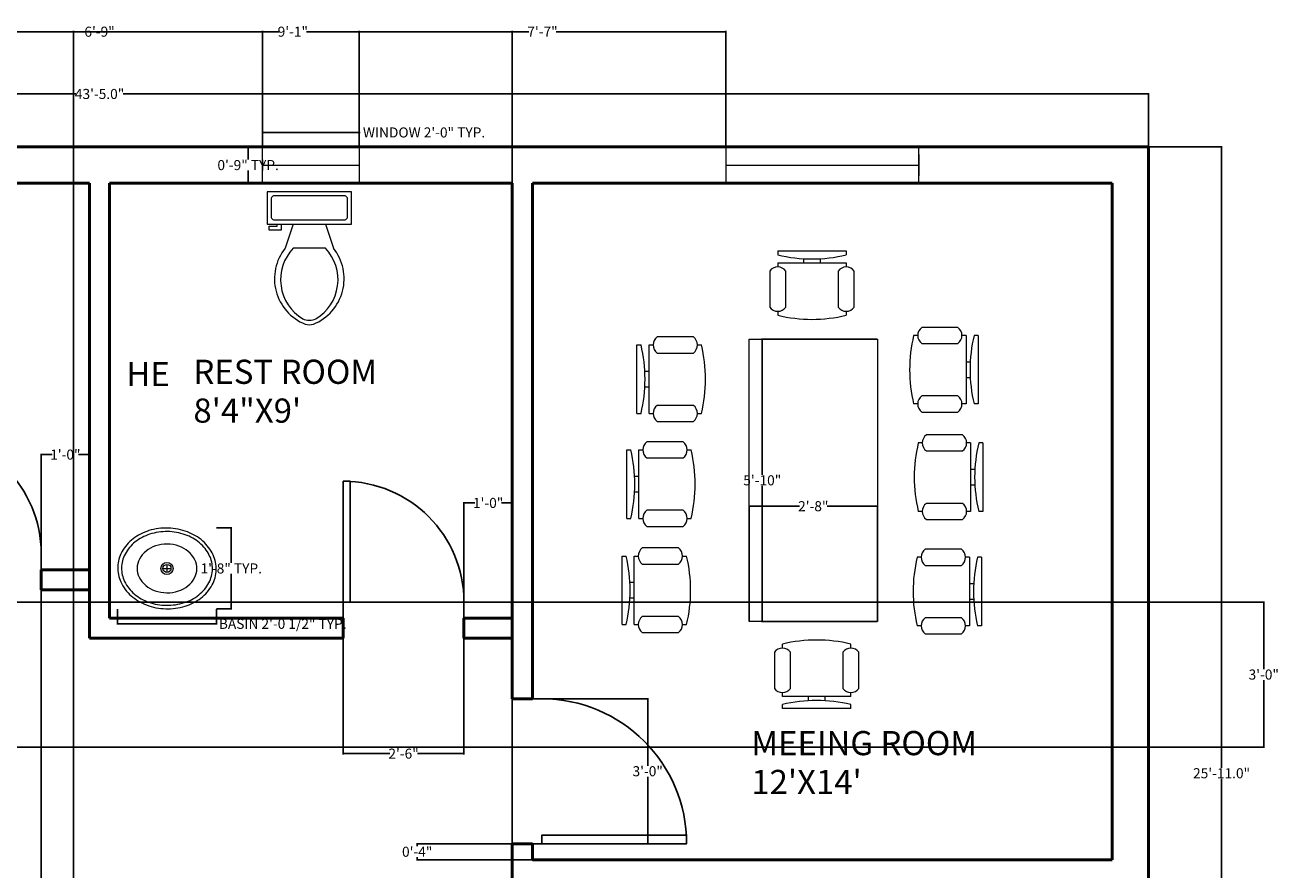
# Model space of a CAD drawing. Units: inches. Extents: x 9441 to 10027, y 18319 to 18830.
# Tile 4 of 4: x 9716 to 10027, y 18618 to 18828. Entities that reach past the tile are written whole.
import ezdxf

# ---------------------------------------------------------------- set-up
doc = ezdxf.new("R2010")
doc.units = ezdxf.units.IN
doc.header["$MEASUREMENT"] = 0
for name, color, linetype, lineweight in [('A-ANNO-DIMS', 2, 'Continuous', 18), ('A-AREA-IDEN', 7, 'Continuous', 25), ('A-DOOR', 3, 'Continuous', 25), ('A-FLOR-FIXT', 9, 'Continuous', 18), ('A-GLAZ', 4, 'Continuous', 18), ('A-WALL', 7, 'Continuous', 50), ('furniture', 8, 'Continuous', 18)]:
    doc.layers.add(name, color=color, linetype=linetype, lineweight=lineweight)
doc.styles.get("Standard").update_dxf_attribs({"font": 'arial.ttf'})
doc.dimstyles.get("Standard").update_dxf_attribs({"dimtxt": 2.5, "dimasz": 0.18, "dimexe": 0.18, "dimexo": 0.0625, "dimgap": 0.09, "dimtad": 0, "dimtih": 1, "dimtoh": 1, "dimdec": 1, "dimzin": 0, "dimdsep": 46, "dimlunit": 3, "dimtxsty": 'Standard', "dimcen": 0.09, "dimadec": 0, "dimazin": 0, "dimtfac": 1, "dimtdec": 1, "dimtofl": 0, "dimtmove": 0, "dimatfit": 3, "dimfxl": 1, "dimtolj": 1, "dimtzin": 0, "dimarcsym": 0})

# ---------------------------------------------------------------- blocks, each defined once
blk = doc.blocks.new('*U2')
for p, q in [((0, 0), (0, -100)), ((750, 0), (750, -100))]:
    blk.add_line(p, q)
blk.add_lwpolyline([(0, 0), (0, 750), (43.75, 750), (43.75, 0)], close=True)
blk.add_arc((0, 0), 750, 0, 90)
blk = doc.blocks.new('*U4')
for p, q in [((0, 100), (0, 0)), ((900, 100), (900, 0)), ((0, 50), (900, 50))]:
    blk.add_line(p, q)
blk = doc.blocks.new('Toilet - top')
for p, q in [((9.5, -6), (9.5, -2)), ((-10, -8.5), (-8, -8.5)), ((-10, -9.5), (-10, -8.5)), ((-8, -8.5), (-8, -8)), ((-7, -8), (-7, -9.5)), ((-4, -8), (-6, -14)), ((4, -8), (6, -14)), ((-7, -9.5), (-10, -9.5)), ((4, -14), (-4, -14))]:
    blk.add_line(p, q)
blk.add_lwpolyline([(10.5, -8), (10.5, 0), (-10.5, 0), (-10.5, -8)], close=True)
for points in [[(-9.5, -2), (-9.5, -6)], [(8.5, -1), (-8.5, -1)], [(-8.5, -7), (8.5, -7)]]:
    blk.add_lwpolyline(points)
for centre, radius, start, end in [((-8.62, -1.88), 0.884, 81.8699, 188.1301), ((8.62, -1.88), 0.884, 351.8699, 98.1301), ((-8.62, -6.12), 0.884, 171.8699, 278.1301), ((8.62, -6.12), 0.884, 261.8699, 8.1301), ((3.52, -21.58), 12.17, 141.4691, 247.9714), ((4.2, -21.82), 11.33, 136.3677, 238.9468), ((-3.52, -21.58), 12.17, 292.0284, 38.5307), ((-4.2, -21.82), 11.33, 301.053, 43.6321), ((0, -27.88), 4, 245.7318, 294.2682), ((0, -29), 4, 254.8605, 285.1395)]:
    blk.add_arc(centre, radius, start, end)
blk = doc.blocks.new('Sink - Oval top')
for p, q in [((-1, 0), (1, 0)), ((0, 1), (0, -1))]:
    blk.add_line(p, q)
for points in [[(-12.23, 0.39, 0.117634), (-11.46, -3.36, 0.104469), (-8.88, -6.8, 0.090016), (-5.08, -9.07, 0.08192), (-0.32, -10.02, 0.08192), (4.49, -9.38, 0.090016), (8.42, -7.36, 0.104469), (11.22, -4.09, 0.117634), (12.23, -0.39, 0.117634), (11.46, 3.36, 0.104469), (8.88, 6.8, 0.090016), (5.08, 9.07, 0.08192), (0.32, 10.02, 0.08192), (-4.49, 9.38, 0.090016), (-8.42, 7.36, 0.104469), (-11.22, 4.09, 0.117634)], [(-11.29, 0.16, 0.118622), (-10.52, -3.25, 0.104678), (-8.07, -6.36, 0.089562), (-4.54, -8.37, 0.081185), (-0.13, -9.15, 0.081185), (4.3, -8.49, 0.089562), (7.89, -6.58, 0.104678), (10.42, -3.55, 0.118622), (11.29, -0.16, 0.118622), (10.52, 3.25, 0.104678), (8.07, 6.36, 0.089562), (4.54, 8.37, 0.081185), (0.13, 9.15, 0.081185), (-4.3, 8.49, 0.089562), (-7.89, 6.58, 0.104678), (-10.42, 3.55, 0.118622)], [(-7.42, 0.08, 0.118283), (-6.91, -2.17, 0.104607), (-5.29, -4.21, 0.089718), (-2.97, -5.53, 0.081436), (-0.07, -6.04, 0.081436), (2.84, -5.59, 0.089718), (5.2, -4.33, 0.104607), (6.86, -2.32, 0.118283), (7.42, -0.08, 0.118283), (6.91, 2.17, 0.104607), (5.29, 4.21, 0.089718), (2.97, 5.53, 0.081436), (0.07, 6.04, 0.081436), (-2.84, 5.59, 0.089718), (-5.2, 4.33, 0.104607), (-6.86, 2.32, 0.118283)]]:
    blk.add_lwpolyline(points, format="xyb", close=True)
for radius in [1.5, 1]:
    blk.add_circle((0, 0), radius)
blk = doc.blocks.new('Chair - Desk')
for p, q in [((-8.5, 0), (-8.5, -1)), ((-8.5, 0), (8.5, 0)), ((8.5, 0), (8.5, -1)), ((-8.5, -3), (-8.5, -4)), ((-8.5, -3), (8.5, -3)), ((-2, -3), (-2, -1.9355)), ((2, -1.9576), (2, -3)), ((8.5, -3), (8.5, -4)), ((-10.5, -5), (-10.5, -14)), ((-6.5, -14), (-6.5, -5)), ((6.5, -5), (6.5, -14)), ((10.5, -14), (10.5, -5)), ((-8.5, -15), (-8.5, -16)), ((8.5, -15), (8.5, -16))]:
    blk.add_line(p, q)
for centre, radius, start, end in [((0, 34.625), 36.625, 256.5803, 283.4197), ((-8.5, -6.5), 2.5, 36.8699, 143.1301), ((8.5, -6.5), 2.5, 36.8699, 143.1301), ((-8.5, -12.5), 2.5, 216.8699, 323.1301), ((8.5, -12.5), 2.5, 216.8699, 323.1301), ((0, 19.625), 36.625, 256.5803, 283.4197)]:
    blk.add_arc(centre, radius, start, end)
blk = doc.blocks.new('*D16')
at = {"layer": 'A-ANNO-DIMS', "color": 0, "lineweight": -2, "transparency": 16777216}
for p, q in [((9473.89, 18797.99), (9473.89, 18811.27)), ((9994.89, 18797.99), (9994.89, 18811.27)), ((9474.07, 18811.09), (9728.5, 18811.09)), ((9994.71, 18811.09), (9740.28, 18811.09))]:
    blk.add_line(p, q, dxfattribs=at)
at = {"layer": 'A-ANNO-DIMS', "color": 0, "transparency": 16777216}
for points in [[(9474.07, 18811.12), (9474.07, 18811.06), (9473.89, 18811.09)], [(9994.71, 18811.12), (9994.71, 18811.06), (9994.89, 18811.09)]]:
    blk.add_solid(points, dxfattribs=at)
at = {"layer": 'Defpoints', "color": 0, "transparency": 16777216}
for p in [(9994.89, 18811.09), (9473.89, 18797.93), (9994.89, 18797.93)]:
    blk.add_point(p, dxfattribs=at)
at = {"layer": 'A-ANNO-DIMS', "color": 0, "transparency": 16777216, "insert": (9734.39, 18811.09), "char_height": 2.5, "attachment_point": 5}
blk.add_mtext('\\A1;43\'-5.0"', dxfattribs=at)
blk = doc.blocks.new('*D17')
at = {"layer": 'A-ANNO-DIMS', "color": 0, "lineweight": -2, "transparency": 16777216}
for p, q in [((9994.95, 18797.93), (10013.22, 18797.93)), ((10013.04, 18797.75), (10013.04, 18643.79)), ((10013.04, 18487.11), (10013.04, 18641.06)), ((9994.95, 18486.93), (10013.22, 18486.93))]:
    blk.add_line(p, q, dxfattribs=at)
at = {"layer": 'A-ANNO-DIMS', "color": 0, "transparency": 16777216}
for points in [[(10013.01, 18797.75), (10013.07, 18797.75), (10013.04, 18797.93)], [(10013.01, 18487.11), (10013.07, 18487.11), (10013.04, 18486.93)]]:
    blk.add_solid(points, dxfattribs=at)
at = {"layer": 'Defpoints', "color": 0, "transparency": 16777216}
for p in [(9994.89, 18797.93), (10013.04, 18797.93), (9994.89, 18486.93)]:
    blk.add_point(p, dxfattribs=at)
at = {"layer": 'A-ANNO-DIMS', "color": 0, "transparency": 16777216, "insert": (10013.04, 18642.43), "char_height": 2.5, "attachment_point": 5}
blk.add_mtext('\\A1;25\'-11.0"', dxfattribs=at)
blk = doc.blocks.new('WIN-FRAME-48x9')
for p, q in [((48, 9), (0, 9)), ((0, 9), (0, 0)), ((48, 0), (48, 9))]:
    blk.add_line(p, q)
blk = doc.blocks.new('WIN-FRAME-24x9')
for p, q in [((0, 0), (0, 9)), ((0, 9), (24, 9)), ((24, 9), (24, 0))]:
    blk.add_line(p, q)
blk = doc.blocks.new('*D27')
at = {"layer": 'A-ANNO-DIMS', "color": 0, "lineweight": -2, "transparency": 16777216}
for p, q in [((9738.85, 18683.15), (9738.85, 18679.35)), ((9763.41, 18683.15), (9763.41, 18679.35)), ((9739.03, 18679.53), (9763.23, 18679.53)), ((9763.41, 18679.53), (9763.59, 18679.53))]:
    blk.add_line(p, q, dxfattribs=at)
at = {"layer": 'A-ANNO-DIMS', "color": 0, "transparency": 16777216}
for points in [[(9739.03, 18679.56), (9739.03, 18679.5), (9738.85, 18679.53)], [(9763.23, 18679.56), (9763.23, 18679.5), (9763.41, 18679.53)]]:
    blk.add_solid(points, dxfattribs=at)
at = {"layer": 'Defpoints', "color": 0, "transparency": 16777216}
for p in [(9738.85, 18683.21), (9763.41, 18683.21), (9763.41, 18679.53)]:
    blk.add_point(p, dxfattribs=at)
at = {"layer": 'A-ANNO-DIMS', "color": 0, "transparency": 16777216, "insert": (9779.88, 18679.53), "char_height": 2.5, "attachment_point": 5}
blk.add_mtext('\\A1;BASIN 2\'-0 1/2" TYP.', dxfattribs=at)
blk = doc.blocks.new('*D28')
at = {"layer": 'A-ANNO-DIMS', "color": 0, "lineweight": -2, "transparency": 16777216}
for p, q in [((9763.47, 18703.35), (9767.27, 18703.35)), ((9767.09, 18703.17), (9767.09, 18694.65)), ((9767.09, 18683.39), (9767.09, 18691.92)), ((9763.47, 18683.21), (9767.27, 18683.21))]:
    blk.add_line(p, q, dxfattribs=at)
at = {"layer": 'A-ANNO-DIMS', "color": 0, "transparency": 16777216}
for points in [[(9767.06, 18703.17), (9767.12, 18703.17), (9767.09, 18703.35)], [(9767.06, 18683.39), (9767.12, 18683.39), (9767.09, 18683.21)]]:
    blk.add_solid(points, dxfattribs=at)
at = {"layer": 'Defpoints', "color": 0, "transparency": 16777216}
for p in [(9763.41, 18703.35), (9767.09, 18703.35), (9763.41, 18683.21)]:
    blk.add_point(p, dxfattribs=at)
at = {"layer": 'A-ANNO-DIMS', "color": 0, "transparency": 16777216, "insert": (9767.09, 18693.28), "char_height": 2.5, "attachment_point": 5}
blk.add_mtext('\\A1;1\'-8" TYP.', dxfattribs=at)
blk = doc.blocks.new('*D29')
at = {"layer": 'A-ANNO-DIMS', "color": 0, "lineweight": -2, "transparency": 16777216}
for p, q in [((9774.89, 18797.99), (9774.89, 18801.71)), ((9775.07, 18801.53), (9798.71, 18801.53)), ((9798.89, 18797.99), (9798.89, 18801.71)), ((9798.89, 18801.53), (9799.07, 18801.53))]:
    blk.add_line(p, q, dxfattribs=at)
at = {"layer": 'A-ANNO-DIMS', "color": 0, "transparency": 16777216}
for points in [[(9775.07, 18801.56), (9775.07, 18801.5), (9774.89, 18801.53)], [(9798.71, 18801.56), (9798.71, 18801.5), (9798.89, 18801.53)]]:
    blk.add_solid(points, dxfattribs=at)
at = {"layer": 'Defpoints', "color": 0, "transparency": 16777216}
for p in [(9798.89, 18801.53), (9774.89, 18797.93), (9798.89, 18797.93)]:
    blk.add_point(p, dxfattribs=at)
at = {"layer": 'A-ANNO-DIMS', "color": 0, "transparency": 16777216, "insert": (9814.98, 18801.53), "char_height": 2.5, "attachment_point": 5}
blk.add_mtext('\\A1;WINDOW 2\'-0" TYP.', dxfattribs=at)
blk = doc.blocks.new('*D30')
at = {"layer": 'A-ANNO-DIMS', "color": 0, "lineweight": -2, "transparency": 16777216}
for p, q in [((9774.83, 18797.93), (9771.11, 18797.93)), ((9771.29, 18797.75), (9771.29, 18794.79)), ((9771.29, 18789.11), (9771.29, 18792.06)), ((9774.83, 18788.93), (9771.11, 18788.93))]:
    blk.add_line(p, q, dxfattribs=at)
at = {"layer": 'A-ANNO-DIMS', "color": 0, "transparency": 16777216}
for points in [[(9771.26, 18797.75), (9771.32, 18797.75), (9771.29, 18797.93)], [(9771.26, 18789.11), (9771.32, 18789.11), (9771.29, 18788.93)]]:
    blk.add_solid(points, dxfattribs=at)
at = {"layer": 'Defpoints', "color": 0, "transparency": 16777216}
for p in [(9771.29, 18797.93), (9774.89, 18797.93), (9774.89, 18788.93)]:
    blk.add_point(p, dxfattribs=at)
at = {"layer": 'A-ANNO-DIMS', "color": 0, "transparency": 16777216, "insert": (9771.29, 18793.43), "char_height": 2.5, "attachment_point": 5}
blk.add_mtext('\\A1;0\'-9" TYP.', dxfattribs=at)
blk = doc.blocks.new('*D43')
at = {"layer": 'A-ANNO-DIMS', "color": 0, "lineweight": -2, "transparency": 16777216}
for p, q in [((9693.89, 18797.99), (9693.89, 18826.73)), ((9694.07, 18826.55), (9730.97, 18826.55)), ((9774.71, 18826.55), (9737.81, 18826.55)), ((9774.89, 18797.99), (9774.89, 18826.73))]:
    blk.add_line(p, q, dxfattribs=at)
at = {"layer": 'A-ANNO-DIMS', "color": 0, "transparency": 16777216}
for points in [[(9694.07, 18826.58), (9694.07, 18826.52), (9693.89, 18826.55)], [(9774.71, 18826.58), (9774.71, 18826.52), (9774.89, 18826.55)]]:
    blk.add_solid(points, dxfattribs=at)
at = {"layer": 'Defpoints', "color": 0, "transparency": 16777216}
for p in [(9774.89, 18826.55), (9693.89, 18797.93), (9774.89, 18797.93)]:
    blk.add_point(p, dxfattribs=at)
at = {"layer": 'A-ANNO-DIMS', "color": 0, "transparency": 16777216, "insert": (9734.39, 18826.55), "char_height": 2.5, "attachment_point": 5}
blk.add_mtext('\\A1;6\'-9"', dxfattribs=at)
blk = doc.blocks.new('*D44')
at = {"layer": 'A-ANNO-DIMS', "color": 0, "lineweight": -2, "transparency": 16777216}
for p, q in [((9798.89, 18797.99), (9798.89, 18826.73)), ((9799.07, 18826.55), (9840.99, 18826.55)), ((9889.71, 18826.55), (9847.79, 18826.55)), ((9889.89, 18797.99), (9889.89, 18826.73))]:
    blk.add_line(p, q, dxfattribs=at)
at = {"layer": 'A-ANNO-DIMS', "color": 0, "transparency": 16777216}
for points in [[(9799.07, 18826.58), (9799.07, 18826.52), (9798.89, 18826.55)], [(9889.71, 18826.58), (9889.71, 18826.52), (9889.89, 18826.55)]]:
    blk.add_solid(points, dxfattribs=at)
at = {"layer": 'Defpoints', "color": 0, "transparency": 16777216}
for p in [(9889.89, 18826.55), (9798.89, 18797.93), (9889.89, 18797.93)]:
    blk.add_point(p, dxfattribs=at)
at = {"layer": 'A-ANNO-DIMS', "color": 0, "transparency": 16777216, "insert": (9844.39, 18826.55), "char_height": 2.5, "attachment_point": 5}
blk.add_mtext('\\A1;7\'-7"', dxfattribs=at)
blk = doc.blocks.new('*D47')
at = {"layer": 'A-ANNO-DIMS', "color": 0, "lineweight": -2, "transparency": 16777216}
for p, q in [((9689.89, 18687.86), (9689.89, 18320.95)), ((9719.89, 18687.86), (9719.89, 18320.95)), ((9690.07, 18321.13), (9701.46, 18321.13)), ((9719.71, 18321.13), (9708.32, 18321.13))]:
    blk.add_line(p, q, dxfattribs=at)
at = {"layer": 'A-ANNO-DIMS', "color": 0, "transparency": 16777216}
for points in [[(9690.07, 18321.16), (9690.07, 18321.1), (9689.89, 18321.13)], [(9719.71, 18321.16), (9719.71, 18321.1), (9719.89, 18321.13)]]:
    blk.add_solid(points, dxfattribs=at)
at = {"layer": 'Defpoints', "color": 0, "transparency": 16777216}
for p in [(9689.89, 18687.93), (9719.89, 18687.93), (9719.89, 18321.13)]:
    blk.add_point(p, dxfattribs=at)
at = {"layer": 'A-ANNO-DIMS', "color": 0, "transparency": 16777216, "insert": (9704.89, 18321.13), "char_height": 2.5, "attachment_point": 5}
blk.add_mtext('\\A1;2\'-6"', dxfattribs=at)
blk = doc.blocks.new('*D48')
at = {"layer": 'A-ANNO-DIMS', "color": 0, "lineweight": -2, "transparency": 16777216}
for p, q in [((9719.89, 18692.99), (9719.89, 18721.73)), ((9720.07, 18721.55), (9722.6, 18721.55)), ((9731.71, 18721.55), (9729.19, 18721.55)), ((9731.89, 18692.99), (9731.89, 18721.73))]:
    blk.add_line(p, q, dxfattribs=at)
at = {"layer": 'A-ANNO-DIMS', "color": 0, "transparency": 16777216}
for points in [[(9720.07, 18721.58), (9720.07, 18721.52), (9719.89, 18721.55)], [(9731.71, 18721.58), (9731.71, 18721.52), (9731.89, 18721.55)]]:
    blk.add_solid(points, dxfattribs=at)
at = {"layer": 'Defpoints', "color": 0, "transparency": 16777216}
for p in [(9731.89, 18721.55), (9719.89, 18692.93), (9731.89, 18692.93)]:
    blk.add_point(p, dxfattribs=at)
at = {"layer": 'A-ANNO-DIMS', "color": 0, "transparency": 16777216, "insert": (9725.89, 18721.55), "char_height": 2.5, "attachment_point": 5}
blk.add_mtext('\\A1;1\'-0"', dxfattribs=at)
blk = doc.blocks.new('*D49')
at = {"layer": 'A-ANNO-DIMS', "color": 0, "lineweight": -2, "transparency": 16777216}
for p, q in [((9794.89, 18675.86), (9794.89, 18647.12)), ((9824.89, 18675.86), (9824.89, 18647.12)), ((9795.07, 18647.3), (9806.46, 18647.3)), ((9824.71, 18647.3), (9813.32, 18647.3))]:
    blk.add_line(p, q, dxfattribs=at)
at = {"layer": 'A-ANNO-DIMS', "color": 0, "transparency": 16777216}
for points in [[(9795.07, 18647.33), (9795.07, 18647.27), (9794.89, 18647.3)], [(9824.71, 18647.33), (9824.71, 18647.27), (9824.89, 18647.3)]]:
    blk.add_solid(points, dxfattribs=at)
at = {"layer": 'Defpoints', "color": 0, "transparency": 16777216}
for p in [(9794.89, 18675.93), (9824.89, 18675.93), (9794.89, 18647.3)]:
    blk.add_point(p, dxfattribs=at)
at = {"layer": 'A-ANNO-DIMS', "color": 0, "transparency": 16777216, "insert": (9809.89, 18647.3), "char_height": 2.5, "attachment_point": 5}
blk.add_mtext('\\A1;2\'-6"', dxfattribs=at)
blk = doc.blocks.new('*D50')
at = {"layer": 'A-ANNO-DIMS', "color": 0, "lineweight": -2, "transparency": 16777216}
for p, q in [((9824.89, 18680.99), (9824.89, 18709.73)), ((9825.07, 18709.55), (9827.6, 18709.55)), ((9836.71, 18709.55), (9834.19, 18709.55)), ((9836.89, 18680.99), (9836.89, 18709.73))]:
    blk.add_line(p, q, dxfattribs=at)
at = {"layer": 'A-ANNO-DIMS', "color": 0, "transparency": 16777216}
for points in [[(9825.07, 18709.58), (9825.07, 18709.52), (9824.89, 18709.55)], [(9836.71, 18709.58), (9836.71, 18709.52), (9836.89, 18709.55)]]:
    blk.add_solid(points, dxfattribs=at)
at = {"layer": 'Defpoints', "color": 0, "transparency": 16777216}
for p in [(9836.89, 18709.55), (9824.89, 18680.93), (9836.89, 18680.93)]:
    blk.add_point(p, dxfattribs=at)
at = {"layer": 'A-ANNO-DIMS', "color": 0, "transparency": 16777216, "insert": (9830.89, 18709.55), "char_height": 2.5, "attachment_point": 5}
blk.add_mtext('\\A1;1\'-0"', dxfattribs=at)
blk = doc.blocks.new('*D51')
at = {"layer": 'A-ANNO-DIMS', "color": 0, "lineweight": -2, "transparency": 16777216}
for p, q in [((9631.95, 18684.93), (10023.7, 18684.93)), ((10023.52, 18684.75), (10023.52, 18668.29)), ((10023.52, 18649.11), (10023.52, 18665.56)), ((9631.95, 18648.93), (10023.7, 18648.93))]:
    blk.add_line(p, q, dxfattribs=at)
at = {"layer": 'A-ANNO-DIMS', "color": 0, "transparency": 16777216}
for points in [[(10023.49, 18684.75), (10023.55, 18684.75), (10023.52, 18684.93)], [(10023.49, 18649.11), (10023.55, 18649.11), (10023.52, 18648.93)]]:
    blk.add_solid(points, dxfattribs=at)
at = {"layer": 'Defpoints', "color": 0, "transparency": 16777216}
for p in [(9631.89, 18684.93), (10023.52, 18684.93), (9631.89, 18648.93)]:
    blk.add_point(p, dxfattribs=at)
at = {"layer": 'A-ANNO-DIMS', "color": 0, "transparency": 16777216, "insert": (10023.52, 18666.93), "char_height": 2.5, "attachment_point": 5}
blk.add_mtext('\\A1;3\'-0"', dxfattribs=at)
blk = doc.blocks.new('*D52')
at = {"layer": 'A-ANNO-DIMS', "color": 0, "lineweight": -2, "transparency": 16777216}
for p, q in [((9841.95, 18660.93), (9870.7, 18660.93)), ((9870.52, 18660.75), (9870.52, 18644.29)), ((9870.52, 18625.11), (9870.52, 18641.56)), ((9841.95, 18624.93), (9870.7, 18624.93))]:
    blk.add_line(p, q, dxfattribs=at)
at = {"layer": 'A-ANNO-DIMS', "color": 0, "transparency": 16777216}
for points in [[(9870.49, 18660.75), (9870.55, 18660.75), (9870.52, 18660.93)], [(9870.49, 18625.11), (9870.55, 18625.11), (9870.52, 18624.93)]]:
    blk.add_solid(points, dxfattribs=at)
at = {"layer": 'Defpoints', "color": 0, "transparency": 16777216}
for p in [(9841.89, 18660.93), (9841.89, 18624.93), (9870.52, 18624.93)]:
    blk.add_point(p, dxfattribs=at)
at = {"layer": 'A-ANNO-DIMS', "color": 0, "transparency": 16777216, "insert": (9870.52, 18642.93), "char_height": 2.5, "attachment_point": 5}
blk.add_mtext('\\A1;3\'-0"', dxfattribs=at)
blk = doc.blocks.new('*D56')
at = {"layer": 'A-ANNO-DIMS', "color": 0, "lineweight": -2, "transparency": 16777216}
for p, q in [((9727.89, 18554.99), (9727.89, 18826.73)), ((9728.07, 18826.55), (9778.98, 18826.55)), ((9836.71, 18826.55), (9785.8, 18826.55)), ((9836.89, 18554.99), (9836.89, 18826.73))]:
    blk.add_line(p, q, dxfattribs=at)
at = {"layer": 'A-ANNO-DIMS', "color": 0, "transparency": 16777216}
for points in [[(9728.07, 18826.58), (9728.07, 18826.52), (9727.89, 18826.55)], [(9836.71, 18826.58), (9836.71, 18826.52), (9836.89, 18826.55)]]:
    blk.add_solid(points, dxfattribs=at)
at = {"layer": 'Defpoints', "color": 0, "transparency": 16777216}
for p in [(9836.89, 18826.55), (9727.89, 18554.93), (9836.89, 18554.93)]:
    blk.add_point(p, dxfattribs=at)
at = {"layer": 'A-ANNO-DIMS', "color": 0, "transparency": 16777216, "insert": (9782.39, 18826.55), "char_height": 2.5, "attachment_point": 5}
blk.add_mtext('\\A1;9\'-1"', dxfattribs=at)
blk = doc.blocks.new('*D62')
at = {"layer": 'A-ANNO-DIMS', "color": 0, "lineweight": -2, "transparency": 16777216}
for p, q in [((9895.7, 18680.17), (9895.7, 18708.91)), ((9895.88, 18708.73), (9908.21, 18708.73)), ((9927.41, 18708.73), (9915.08, 18708.73)), ((9927.59, 18680.17), (9927.59, 18708.91))]:
    blk.add_line(p, q, dxfattribs=at)
at = {"layer": 'A-ANNO-DIMS', "color": 0, "transparency": 16777216}
for points in [[(9895.88, 18708.76), (9895.88, 18708.7), (9895.7, 18708.73)], [(9927.41, 18708.76), (9927.41, 18708.7), (9927.59, 18708.73)]]:
    blk.add_solid(points, dxfattribs=at)
at = {"layer": 'Defpoints', "color": 0, "transparency": 16777216}
for p in [(9927.59, 18708.73), (9895.7, 18680.1), (9927.59, 18680.1)]:
    blk.add_point(p, dxfattribs=at)
at = {"layer": 'A-ANNO-DIMS', "color": 0, "transparency": 16777216, "insert": (9911.64, 18708.73), "char_height": 2.5, "attachment_point": 5}
blk.add_mtext('\\A1;2\'-8"', dxfattribs=at)
blk = doc.blocks.new('*D63')
at = {"layer": 'A-ANNO-DIMS', "color": 0, "lineweight": -2, "transparency": 16777216}
for p, q in [((9927.53, 18750.22), (9898.79, 18750.22)), ((9898.97, 18750.04), (9898.97, 18716.53)), ((9898.97, 18680.28), (9898.97, 18713.8)), ((9927.53, 18680.1), (9898.79, 18680.1))]:
    blk.add_line(p, q, dxfattribs=at)
at = {"layer": 'A-ANNO-DIMS', "color": 0, "transparency": 16777216}
for points in [[(9898.94, 18750.04), (9899, 18750.04), (9898.97, 18750.22)], [(9898.94, 18680.28), (9899, 18680.28), (9898.97, 18680.1)]]:
    blk.add_solid(points, dxfattribs=at)
at = {"layer": 'Defpoints', "color": 0, "transparency": 16777216}
for p in [(9898.97, 18750.22), (9927.59, 18750.22), (9927.59, 18680.1)]:
    blk.add_point(p, dxfattribs=at)
at = {"layer": 'A-ANNO-DIMS', "color": 0, "transparency": 16777216, "insert": (9898.97, 18715.16), "char_height": 2.5, "attachment_point": 5}
blk.add_mtext('\\A1;5\'-10"', dxfattribs=at)
blk = doc.blocks.new('*D72')
at = {"layer": 'A-ANNO-DIMS', "color": 0, "lineweight": -2, "transparency": 16777216}
for p, q in [((9841.83, 18624.93), (9813.09, 18624.93)), ((9813.27, 18624.75), (9813.27, 18624.29)), ((9813.27, 18621.11), (9813.27, 18621.56)), ((9841.83, 18620.93), (9813.09, 18620.93))]:
    blk.add_line(p, q, dxfattribs=at)
at = {"layer": 'A-ANNO-DIMS', "color": 0, "transparency": 16777216}
for points in [[(9813.24, 18624.75), (9813.3, 18624.75), (9813.27, 18624.93)], [(9813.24, 18621.11), (9813.3, 18621.11), (9813.27, 18620.93)]]:
    blk.add_solid(points, dxfattribs=at)
at = {"layer": 'Defpoints', "color": 0, "transparency": 16777216}
for p in [(9813.27, 18624.93), (9841.89, 18624.93), (9841.89, 18620.93)]:
    blk.add_point(p, dxfattribs=at)
at = {"layer": 'A-ANNO-DIMS', "color": 0, "transparency": 16777216, "insert": (9813.27, 18622.93), "char_height": 2.5, "attachment_point": 5}
blk.add_mtext('\\A1;0\'-4"', dxfattribs=at)

msp = doc.modelspace()

# ---------------------------------------------------------------- linework, layer by layer
at = {"layer": 'A-WALL'}
for p, q in [((9473.89, 18797.93), (9994.89, 18797.93)), ((9994.89, 18486.93), (9994.89, 18797.93)), ((9631.89, 18788.93), (9731.89, 18788.93)), ((9731.89, 18675.93), (9731.89, 18788.93)), ((9736.89, 18680.93), (9736.89, 18788.93)), ((9736.89, 18788.93), (9836.89, 18788.93)), ((9836.89, 18660.93), (9836.89, 18788.93)), ((9841.89, 18660.93), (9841.89, 18788.93)), ((9841.89, 18788.93), (9985.89, 18788.93)), ((9985.89, 18620.93), (9985.89, 18788.93)), ((9719.89, 18692.93), (9719.89, 18687.93)), ((9719.89, 18692.93), (9731.89, 18692.93)), ((9719.89, 18687.93), (9731.89, 18687.93)), ((9736.89, 18680.93), (9794.89, 18680.93)), ((9794.89, 18675.93), (9794.89, 18680.93)), ((9824.89, 18680.93), (9824.89, 18675.93)), ((9824.89, 18680.93), (9836.89, 18680.93)), ((9731.89, 18675.93), (9794.89, 18675.93)), ((9824.89, 18675.93), (9836.89, 18675.93)), ((9836.89, 18660.93), (9841.89, 18660.93)), ((9841.89, 18624.93), (9836.89, 18624.93)), ((9836.89, 18611.93), (9836.89, 18624.93)), ((9841.89, 18620.93), (9841.89, 18624.93)), ((9841.89, 18620.93), (9985.89, 18620.93))]:
    msp.add_line(p, q, dxfattribs=at)
at = {"layer": 'furniture'}
msp.add_lwpolyline([(9895.7, 18750.22), (9927.59, 18750.22), (9927.59, 18680.1), (9895.7, 18680.1)], close=True, dxfattribs=at)

# ---------------------------------------------------------------- block references
at = {"layer": 'A-DOOR', "xscale": 0.0400000000000005, "yscale": 0.0400000000000005, "zscale": 0.0400000000000005}
for p in [(9689.89, 18696.93), (9794.89, 18684.93)]:
    msp.add_blockref('*U2', p, dxfattribs=at)
at = {"layer": 'A-DOOR', "xscale": -0.0480000000000006, "yscale": 0.0480000000000006, "zscale": 0.0480000000000006, "rotation": 270}
msp.add_blockref('*U2', (9844.19, 18624.93), dxfattribs=at)
at = {"layer": 'A-FLOR-FIXT'}
for name, p in [('Toilet - top', (9786.48, 18786.8)), ('Sink - Oval top', (9751.13, 18693.28))]:
    msp.add_blockref(name, p, dxfattribs=at)
at = {"layer": 'A-GLAZ'}
for name, p in [('WIN-FRAME-24x9', (9774.89, 18788.93)), ('WIN-FRAME-48x9', (9889.89, 18788.93))]:
    msp.add_blockref(name, p, dxfattribs=at)
for p, xscale, yscale, zscale in [((9889.89, 18790.76), 0.0533333333333332, 0.0533333333333332, 0.0533333333333332), ((9774.89, 18792.09), 0.0266666666666666, 0.0266666666666666, 0.0266666666666666)]:
    msp.add_blockref('*U4', p, dxfattribs=dict(at, xscale=xscale, yscale=yscale, zscale=zscale))
at = {"layer": 'furniture'}
msp.add_blockref('Chair - Desk', (9911.31, 18772.13), dxfattribs=at)
for p, rotation in [((9952.57, 18742.62), 270), ((9867.86, 18740.27), 90), ((9865.31, 18714.21), 90), ((9953.72, 18715.94), 270), ((9864.18, 18687.86), 90), ((9953.43, 18687.54), 270), ((9912.47, 18658.5), 180)]:
    msp.add_blockref('Chair - Desk', p, dxfattribs=dict(at, rotation=rotation))

# ---------------------------------------------------------------- texts
at = {"layer": 'A-AREA-IDEN'}
for s, p in [('HE', (9741.06, 18738.54)), ('REST ROOM', (9757.7, 18739.11)), ('8\'4"X9\'', (9757.7, 18729.47)), ('MEEING ROOM', (9896.25, 18646.91)), ("12'X14'", (9896.25, 18637.27))]:
    msp.add_text(s, height=6, dxfattribs=at).set_placement(p)

# ---------------------------------------------------------------- dimensions: what is measured, and where the dimension line sits
at = {"layer": 'A-ANNO-DIMS'}
for base, p1, p2, override, picture, middle in [((9774.89, 18826.55), (9693.89, 18797.93), (9774.89, 18797.93), {"dimdec": 1, "dimlfac": 1, "dimrnd": 0, "dimzin": 1, "dimdsep": 46, "dimlunit": 4, "dimfrac": 2}, '*D43', (9734.39, 18826.55)), ((9836.89, 18826.55), (9727.89, 18554.93), (9836.89, 18554.93), {"dimdec": 1, "dimlfac": 1, "dimrnd": 0, "dimzin": 1, "dimdsep": 46, "dimlunit": 4, "dimfrac": 2}, '*D56', (9782.39, 18826.55)), ((9889.89, 18826.55), (9798.89, 18797.93), (9889.89, 18797.93), {"dimdec": 1, "dimlfac": 1, "dimrnd": 0, "dimzin": 1, "dimdsep": 46, "dimlunit": 4, "dimfrac": 2}, '*D44', (9844.39, 18826.55)), ((9994.89, 18811.09), (9473.89, 18797.93), (9994.89, 18797.93), {"dimclrd": 0, "dimclre": 0, "dimclrt": 0}, '*D16', (9734.39, 18811.09)), ((9731.89, 18721.55), (9719.89, 18692.93), (9731.89, 18692.93), {"dimdec": 1, "dimlfac": 1, "dimrnd": 0, "dimzin": 1, "dimdsep": 46, "dimlunit": 4, "dimfrac": 2}, '*D48', (9725.89, 18721.55)), ((9836.89, 18709.55), (9824.89, 18680.93), (9836.89, 18680.93), {"dimdec": 1, "dimlfac": 1, "dimrnd": 0, "dimzin": 1, "dimdsep": 46, "dimlunit": 4, "dimfrac": 2}, '*D50', (9830.89, 18709.55)), ((9927.59, 18708.73), (9895.7, 18680.1), (9927.59, 18680.1), {"dimdec": 1, "dimlfac": 1, "dimrnd": 0, "dimzin": 1, "dimdsep": 46, "dimlunit": 4, "dimfrac": 2}, '*D62', (9911.64, 18708.73)), ((9719.89, 18321.13), (9689.89, 18687.93), (9719.89, 18687.93), {"dimdec": 1, "dimlfac": 1, "dimrnd": 0, "dimzin": 1, "dimdsep": 46, "dimlunit": 4, "dimfrac": 2}, '*D47', (9704.89, 18321.13))]:
    dim = msp.add_linear_dim(base=base, p1=p1, p2=p2, dimstyle='Standard', override=override, dxfattribs=at)
    dim.commit()
    dim.dimension.update_dxf_attribs({"geometry": picture, "text_midpoint": middle})
for base, p1, p2, text, picture, middle in [((9798.89, 18801.53), (9774.89, 18797.93), (9798.89, 18797.93), 'WINDOW <> TYP.', '*D29', (9814.98, 18801.53)), ((9763.41, 18679.53), (9738.85, 18683.21), (9763.41, 18683.21), 'BASIN <> TYP.', '*D27', (9779.88, 18679.53))]:
    dim = msp.add_linear_dim(base=base, p1=p1, p2=p2, text=text, dimstyle='Standard', override={"dimdec": 1, "dimlfac": 1, "dimrnd": 0, "dimzin": 1, "dimdsep": 46, "dimlunit": 4, "dimfrac": 2}, dxfattribs=at)
    dim.commit()
    dim.dimension.update_dxf_attribs({"geometry": picture, "text_midpoint": middle})
for base, p1, p2, picture, middle in [((9771.29, 18797.93), (9774.89, 18788.93), (9774.89, 18797.93), '*D30', (9771.29, 18793.43)), ((9767.09, 18703.35), (9763.41, 18683.21), (9763.41, 18703.35), '*D28', (9767.09, 18693.28))]:
    dim = msp.add_linear_dim(base=base, p1=p1, p2=p2, angle=90, text='<> TYP.', dimstyle='Standard', override={"dimdec": 1, "dimlfac": 1, "dimrnd": 0, "dimzin": 1, "dimdsep": 46, "dimlunit": 4, "dimfrac": 2}, dxfattribs=at)
    dim.commit()
    dim.dimension.update_dxf_attribs({"geometry": picture, "text_midpoint": middle})
for base, p1, p2, angle, override, picture, middle in [((10013.04, 18797.93), (9994.89, 18486.93), (9994.89, 18797.93), 90, {"dimclrd": 0, "dimclre": 0, "dimclrt": 0}, '*D17', (10013.04, 18642.43)), ((9898.97, 18750.22), (9927.59, 18680.1), (9927.59, 18750.22), 90, {"dimdec": 1, "dimlfac": 1, "dimrnd": 0, "dimzin": 1, "dimdsep": 46, "dimlunit": 4, "dimfrac": 2}, '*D63', (9898.97, 18715.16)), ((10023.52, 18684.93), (9631.89, 18648.93), (9631.89, 18684.93), 90, {"dimdec": 1, "dimlfac": 1, "dimrnd": 0, "dimzin": 1, "dimdsep": 46, "dimlunit": 4, "dimfrac": 2}, '*D51', (10023.52, 18666.93)), ((9794.89, 18647.3), (9824.89, 18675.93), (9794.89, 18675.93), 180, {"dimdec": 1, "dimlfac": 1, "dimrnd": 0, "dimzin": 1, "dimdsep": 46, "dimlunit": 4, "dimfrac": 2}, '*D49', (9809.89, 18647.3)), ((9870.52, 18624.93), (9841.89, 18660.93), (9841.89, 18624.93), 270, {"dimdec": 1, "dimlfac": 1, "dimrnd": 0, "dimzin": 1, "dimdsep": 46, "dimlunit": 4, "dimfrac": 2}, '*D52', (9870.52, 18642.93)), ((9813.27, 18624.93), (9841.89, 18620.93), (9841.89, 18624.93), 90, {"dimdec": 1, "dimlfac": 1, "dimrnd": 0, "dimzin": 1, "dimdsep": 46, "dimlunit": 4, "dimfrac": 2}, '*D72', (9813.27, 18622.93))]:
    dim = msp.add_linear_dim(base=base, p1=p1, p2=p2, angle=angle, dimstyle='Standard', override=override, dxfattribs=at)
    dim.commit()
    dim.dimension.update_dxf_attribs({"geometry": picture, "text_midpoint": middle})

doc.saveas('drawing.dxf')
